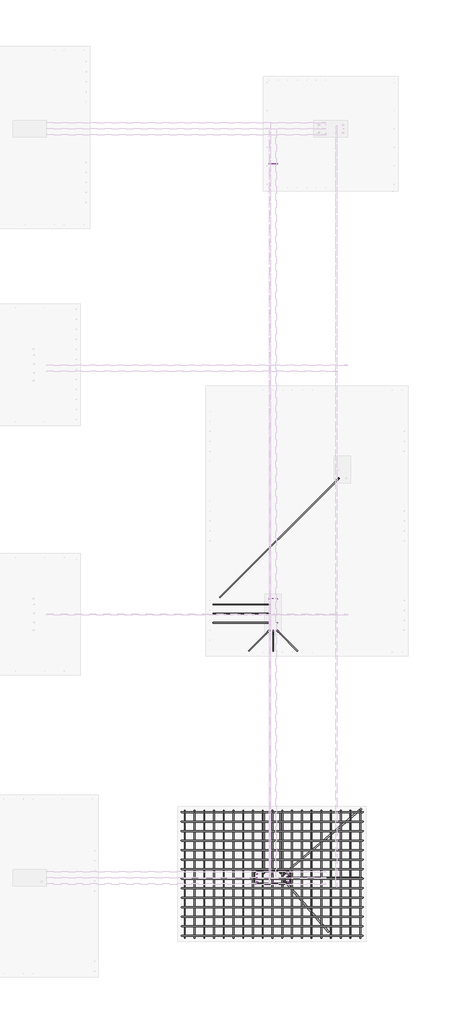
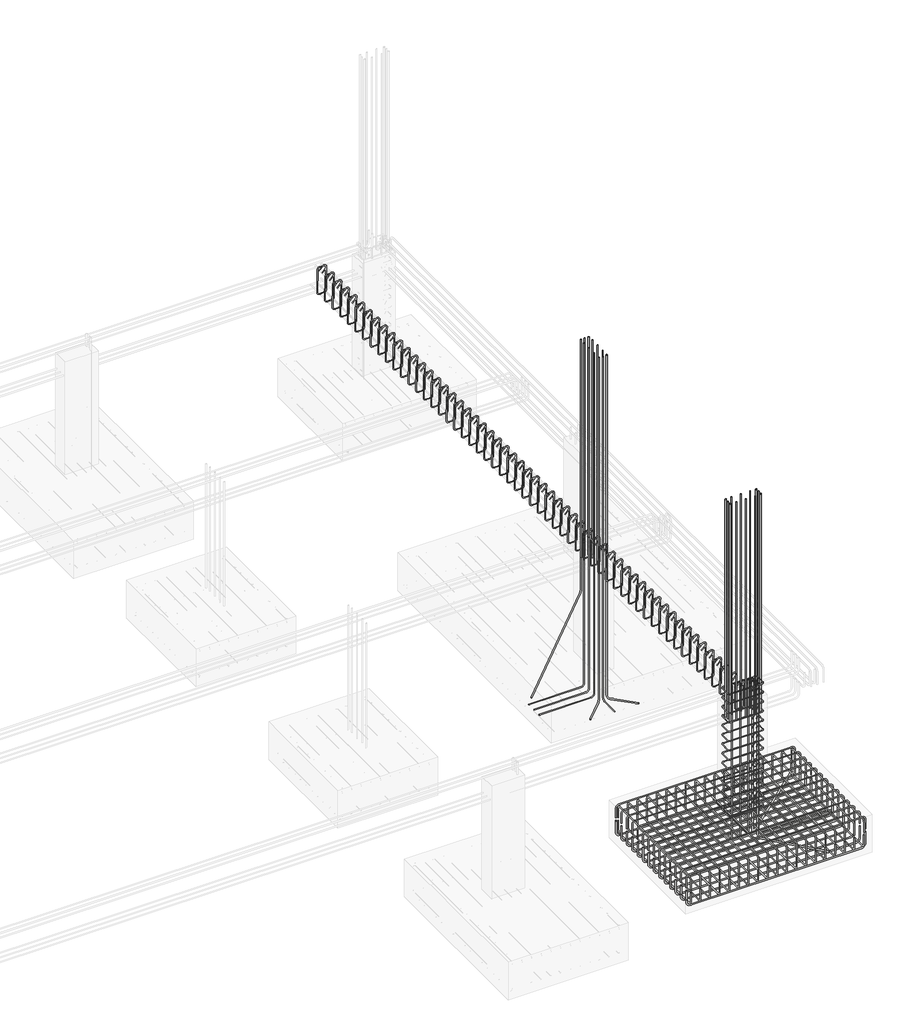
# One storey, part 9 of 18: 31 reinforcing bars.
"""IFC4 building model written with IfcOpenShell, lengths in millimetres."""

from ifc_helpers import new_model, si_unit, point, frame, origin, place, context, project, spatial, polyline, circle_curve, trimmed, segment, composite_curve, source, transform, mapped, element, save
from ifc_brep_helpers import swept_disk

model = new_model("IFC4")

# Units and contexts
model_context = context("Model", 3, world=origin())
ifc_project = project(units=[si_unit("LENGTHUNIT", "METRE", prefix="MILLI")], contexts=[model_context])

# Site, building, storey
site = spatial("IfcSite", under=ifc_project)
building = spatial("IfcBuilding", under=site)
storey = spatial("IfcBuildingStorey", under=building, Elevation=-2000.0)

# Reinforcing bars
placement = place(None, origin())
reinforcing_bar_shape = source(origin(), model_context, "Body", "SolidModel", [
    swept_disk(composite_curve([segment(polyline([(10867.920951, -4585.2975898, -2300.0), (10867.920951, -4585.2975898, -2486.6)]), True, "CONTINUOUS"), segment(trimmed(circle_curve(frame((10812.470951, -4585.2975898, -2486.6), z_axis=(0.0, 1.0, 0.0), x_axis=(55.45000000000073, 0.0, 0.0)), 55.45), [point((10867.920951, -4585.2975898, -2486.6))], [point((10812.470951, -4585.2975898, -2542.05))], True, "CARTESIAN"), True, "CONTINUOUS"), segment(polyline([(10812.470951, -4585.2975898, -2542.05), (8239.270951, -4585.2975898, -2542.05)]), True, "CONTINUOUS"), segment(trimmed(circle_curve(frame((8239.270951, -4585.2975898, -2486.6), z_axis=(0.0, 1.0, 0.0), x_axis=(0.0, 0.0, -55.45000000000027)), 55.45), [point((8239.270951, -4585.2975898, -2542.05))], [point((8183.820951, -4585.2975898, -2486.6))], True, "CARTESIAN"), True, "CONTINUOUS"), segment(polyline([(8183.820951, -4585.2975898, -2486.6), (8183.820951, -4585.2975898, -2300.0)]), True, "CONTINUOUS")], self_intersect=False), 7.95),
])
element("IfcReinforcingBar", 1, at=placement, inside=storey, context=model_context, shape_type="MappedRepresentation", body=[
    mapped(reinforcing_bar_shape, transform((0.0, 0.0, 0.0), x_axis=(1.0, 0.0, 0.0), y_axis=(0.0, 1.0, 0.0), z_axis=(0.0, 0.0, 1.0))),
    mapped(reinforcing_bar_shape, transform((0.0, -140.97506, 0.0), x_axis=(1.0, 0.0, 0.0), y_axis=(0.0, 1.0, 0.0), z_axis=(0.0, 0.0, 1.0))),
    mapped(reinforcing_bar_shape, transform((0.0, -281.9501199, 0.0), x_axis=(1.0, 0.0, 0.0), y_axis=(0.0, 1.0, 0.0), z_axis=(0.0, 0.0, 1.0))),
    mapped(reinforcing_bar_shape, transform((0.0, -422.9251799, 0.0), x_axis=(1.0, 0.0, 0.0), y_axis=(0.0, 1.0, 0.0), z_axis=(0.0, 0.0, 1.0))),
    mapped(reinforcing_bar_shape, transform((0.0, -563.9002399, 0.0), x_axis=(1.0, 0.0, 0.0), y_axis=(0.0, 1.0, 0.0), z_axis=(0.0, 0.0, 1.0))),
    mapped(reinforcing_bar_shape, transform((0.0, -704.8752999, 0.0), x_axis=(1.0, 0.0, 0.0), y_axis=(0.0, 1.0, 0.0), z_axis=(0.0, 0.0, 1.0))),
    mapped(reinforcing_bar_shape, transform((0.0, -845.8503598, 0.0), x_axis=(1.0, 0.0, 0.0), y_axis=(0.0, 1.0, 0.0), z_axis=(0.0, 0.0, 1.0))),
    mapped(reinforcing_bar_shape, transform((0.0, -986.8254198, 0.0), x_axis=(1.0, 0.0, 0.0), y_axis=(0.0, 1.0, 0.0), z_axis=(0.0, 0.0, 1.0))),
    mapped(reinforcing_bar_shape, transform((0.0, -1127.8004798, 0.0), x_axis=(1.0, 0.0, 0.0), y_axis=(0.0, 1.0, 0.0), z_axis=(0.0, 0.0, 1.0))),
    mapped(reinforcing_bar_shape, transform((0.0, -1268.7755397, 0.0), x_axis=(1.0, 0.0, 0.0), y_axis=(0.0, 1.0, 0.0), z_axis=(0.0, 0.0, 1.0))),
    mapped(reinforcing_bar_shape, transform((0.0, -1409.7505997, 0.0), x_axis=(1.0, 0.0, 0.0), y_axis=(0.0, 1.0, 0.0), z_axis=(0.0, 0.0, 1.0))),
    mapped(reinforcing_bar_shape, transform((0.0, -1550.7256597, 0.0), x_axis=(1.0, 0.0, 0.0), y_axis=(0.0, 1.0, 0.0), z_axis=(0.0, 0.0, 1.0))),
    mapped(reinforcing_bar_shape, transform((0.0, -1691.7007197, 0.0), x_axis=(1.0, 0.0, 0.0), y_axis=(0.0, 1.0, 0.0), z_axis=(0.0, 0.0, 1.0))),
    mapped(reinforcing_bar_shape, transform((0.0, -1832.6757796, 0.0), x_axis=(1.0, 0.0, 0.0), y_axis=(0.0, 1.0, 0.0), z_axis=(0.0, 0.0, 1.0))),
])
reinforcing_bar_2_shape = source(origin(), model_context, "Body", "SolidModel", [
    swept_disk(composite_curve([segment(polyline([(8181.870951, -4585.2975898, -2250.0), (8181.870951, -4585.2975898, -2102.0)]), True, "CONTINUOUS"), segment(trimmed(circle_curve(frame((8227.870951, -4585.2975898, -2102.0), z_axis=(0.0, 1.0, 0.0), x_axis=(-46.00000000000091, 0.0, 0.0)), 46.0), [point((8181.870951, -4585.2975898, -2102.0))], [point((8227.870951, -4585.2975898, -2056.0))], True, "CARTESIAN"), True, "CONTINUOUS"), segment(polyline([(8227.870951, -4585.2975898, -2056.0), (10823.870951, -4585.2975898, -2056.0)]), True, "CONTINUOUS"), segment(trimmed(circle_curve(frame((10823.870951, -4585.2975898, -2102.0), z_axis=(0.0, 1.0, 0.0), x_axis=(0.0, 0.0, 46.0)), 46.0), [point((10823.870951, -4585.2975898, -2056.0))], [point((10869.870951, -4585.2975898, -2102.0))], True, "CARTESIAN"), True, "CONTINUOUS"), segment(polyline([(10869.870951, -4585.2975898, -2102.0), (10869.870951, -4585.2975898, -2250.0)]), True, "CONTINUOUS")], self_intersect=False), 6.0),
])
element("IfcReinforcingBar", 2, at=placement, inside=storey, context=model_context, shape_type="MappedRepresentation", body=[
    mapped(reinforcing_bar_2_shape, transform((0.0, 0.0, 0.0), x_axis=(1.0, 0.0, 0.0), y_axis=(0.0, 1.0, 0.0), z_axis=(0.0, 0.0, 1.0))),
    mapped(reinforcing_bar_2_shape, transform((0.0, -140.97506, 0.0), x_axis=(1.0, 0.0, 0.0), y_axis=(0.0, 1.0, 0.0), z_axis=(0.0, 0.0, 1.0))),
    mapped(reinforcing_bar_2_shape, transform((0.0, -281.9501199, 0.0), x_axis=(1.0, 0.0, 0.0), y_axis=(0.0, 1.0, 0.0), z_axis=(0.0, 0.0, 1.0))),
    mapped(reinforcing_bar_2_shape, transform((0.0, -422.9251799, 0.0), x_axis=(1.0, 0.0, 0.0), y_axis=(0.0, 1.0, 0.0), z_axis=(0.0, 0.0, 1.0))),
    mapped(reinforcing_bar_2_shape, transform((0.0, -563.9002399, 0.0), x_axis=(1.0, 0.0, 0.0), y_axis=(0.0, 1.0, 0.0), z_axis=(0.0, 0.0, 1.0))),
    mapped(reinforcing_bar_2_shape, transform((0.0, -704.8752999, 0.0), x_axis=(1.0, 0.0, 0.0), y_axis=(0.0, 1.0, 0.0), z_axis=(0.0, 0.0, 1.0))),
    mapped(reinforcing_bar_2_shape, transform((0.0, -845.8503598, 0.0), x_axis=(1.0, 0.0, 0.0), y_axis=(0.0, 1.0, 0.0), z_axis=(0.0, 0.0, 1.0))),
    mapped(reinforcing_bar_2_shape, transform((0.0, -986.8254198, 0.0), x_axis=(1.0, 0.0, 0.0), y_axis=(0.0, 1.0, 0.0), z_axis=(0.0, 0.0, 1.0))),
    mapped(reinforcing_bar_2_shape, transform((0.0, -1127.8004798, 0.0), x_axis=(1.0, 0.0, 0.0), y_axis=(0.0, 1.0, 0.0), z_axis=(0.0, 0.0, 1.0))),
    mapped(reinforcing_bar_2_shape, transform((0.0, -1268.7755397, 0.0), x_axis=(1.0, 0.0, 0.0), y_axis=(0.0, 1.0, 0.0), z_axis=(0.0, 0.0, 1.0))),
    mapped(reinforcing_bar_2_shape, transform((0.0, -1409.7505997, 0.0), x_axis=(1.0, 0.0, 0.0), y_axis=(0.0, 1.0, 0.0), z_axis=(0.0, 0.0, 1.0))),
    mapped(reinforcing_bar_2_shape, transform((0.0, -1550.7256597, 0.0), x_axis=(1.0, 0.0, 0.0), y_axis=(0.0, 1.0, 0.0), z_axis=(0.0, 0.0, 1.0))),
    mapped(reinforcing_bar_2_shape, transform((0.0, -1691.7007197, 0.0), x_axis=(1.0, 0.0, 0.0), y_axis=(0.0, 1.0, 0.0), z_axis=(0.0, 0.0, 1.0))),
    mapped(reinforcing_bar_2_shape, transform((0.0, -1832.6757796, 0.0), x_axis=(1.0, 0.0, 0.0), y_axis=(0.0, 1.0, 0.0), z_axis=(0.0, 0.0, 1.0))),
])
reinforcing_bar_3_shape = source(origin(), model_context, "Body", "SolidModel", [
    swept_disk(composite_curve([segment(polyline([(8228.0517338, -4562.4021146, -2322.6684255), (8228.0517338, -4562.4021146, -2470.6684255)]), True, "CONTINUOUS"), segment(trimmed(circle_curve(frame((8228.0517338, -4608.4021146, -2470.6684255), z_axis=(-1.0, 0.0, 0.0), x_axis=(0.0, 46.0, 0.0)), 46.0), [point((8228.0517338, -4562.4021146, -2470.6684255))], [point((8228.0517338, -4608.4021146, -2516.6684255))], True, "CARTESIAN"), True, "CONTINUOUS"), segment(polyline([(8228.0517338, -4608.4021146, -2516.6684255), (8228.0517338, -6404.4021146, -2516.6684255)]), True, "CONTINUOUS"), segment(trimmed(circle_curve(frame((8228.0517338, -6404.4021146, -2470.6684255), z_axis=(-1.0, 0.0, 0.0), x_axis=(0.0, 0.0, -46.0)), 46.0), [point((8228.0517338, -6404.4021146, -2516.6684255))], [point((8228.0517338, -6450.4021146, -2470.6684255))], True, "CARTESIAN"), True, "CONTINUOUS"), segment(polyline([(8228.0517338, -6450.4021146, -2470.6684255), (8228.0517338, -6450.4021146, -2322.6684255)]), True, "CONTINUOUS")], self_intersect=False), 6.0),
])
element("IfcReinforcingBar", 3, at=placement, inside=storey, context=model_context, shape_type="MappedRepresentation", body=[
    mapped(reinforcing_bar_3_shape, transform((0.0, 0.0, 0.0), x_axis=(1.0, 0.0, 0.0), y_axis=(0.0, 1.0, 0.0), z_axis=(0.0, 0.0, 1.0))),
    mapped(reinforcing_bar_3_shape, transform((144.6566146, 0.0, 0.0), x_axis=(1.0, 0.0, 0.0), y_axis=(0.0, 1.0, 0.0), z_axis=(0.0, 0.0, 1.0))),
    mapped(reinforcing_bar_3_shape, transform((289.3132291, 0.0, 0.0), x_axis=(1.0, 0.0, 0.0), y_axis=(0.0, 1.0, 0.0), z_axis=(0.0, 0.0, 1.0))),
    mapped(reinforcing_bar_3_shape, transform((433.9698437, 0.0, 0.0), x_axis=(1.0, 0.0, 0.0), y_axis=(0.0, 1.0, 0.0), z_axis=(0.0, 0.0, 1.0))),
    mapped(reinforcing_bar_3_shape, transform((578.6264583, 0.0, 0.0), x_axis=(1.0, 0.0, 0.0), y_axis=(0.0, 1.0, 0.0), z_axis=(0.0, 0.0, 1.0))),
    mapped(reinforcing_bar_3_shape, transform((723.2830729, 0.0, 0.0), x_axis=(1.0, 0.0, 0.0), y_axis=(0.0, 1.0, 0.0), z_axis=(0.0, 0.0, 1.0))),
    mapped(reinforcing_bar_3_shape, transform((867.9396874, 0.0, 0.0), x_axis=(1.0, 0.0, 0.0), y_axis=(0.0, 1.0, 0.0), z_axis=(0.0, 0.0, 1.0))),
    mapped(reinforcing_bar_3_shape, transform((1012.596302, 0.0, 0.0), x_axis=(1.0, 0.0, 0.0), y_axis=(0.0, 1.0, 0.0), z_axis=(0.0, 0.0, 1.0))),
    mapped(reinforcing_bar_3_shape, transform((1157.2529166, 0.0, 0.0), x_axis=(1.0, 0.0, 0.0), y_axis=(0.0, 1.0, 0.0), z_axis=(0.0, 0.0, 1.0))),
    mapped(reinforcing_bar_3_shape, transform((1301.9095312, 0.0, 0.0), x_axis=(1.0, 0.0, 0.0), y_axis=(0.0, 1.0, 0.0), z_axis=(0.0, 0.0, 1.0))),
    mapped(reinforcing_bar_3_shape, transform((1446.5661457, 0.0, 0.0), x_axis=(1.0, 0.0, 0.0), y_axis=(0.0, 1.0, 0.0), z_axis=(0.0, 0.0, 1.0))),
    mapped(reinforcing_bar_3_shape, transform((1591.2227603, 0.0, 0.0), x_axis=(1.0, 0.0, 0.0), y_axis=(0.0, 1.0, 0.0), z_axis=(0.0, 0.0, 1.0))),
    mapped(reinforcing_bar_3_shape, transform((1735.8793749, 0.0, 0.0), x_axis=(1.0, 0.0, 0.0), y_axis=(0.0, 1.0, 0.0), z_axis=(0.0, 0.0, 1.0))),
    mapped(reinforcing_bar_3_shape, transform((1880.5359895, 0.0, 0.0), x_axis=(1.0, 0.0, 0.0), y_axis=(0.0, 1.0, 0.0), z_axis=(0.0, 0.0, 1.0))),
    mapped(reinforcing_bar_3_shape, transform((2025.192604, 0.0, 0.0), x_axis=(1.0, 0.0, 0.0), y_axis=(0.0, 1.0, 0.0), z_axis=(0.0, 0.0, 1.0))),
    mapped(reinforcing_bar_3_shape, transform((2169.8492186, 0.0, 0.0), x_axis=(1.0, 0.0, 0.0), y_axis=(0.0, 1.0, 0.0), z_axis=(0.0, 0.0, 1.0))),
    mapped(reinforcing_bar_3_shape, transform((2314.5058332, 0.0, 0.0), x_axis=(1.0, 0.0, 0.0), y_axis=(0.0, 1.0, 0.0), z_axis=(0.0, 0.0, 1.0))),
    mapped(reinforcing_bar_3_shape, transform((2459.1624478, 0.0, 0.0), x_axis=(1.0, 0.0, 0.0), y_axis=(0.0, 1.0, 0.0), z_axis=(0.0, 0.0, 1.0))),
    mapped(reinforcing_bar_3_shape, transform((2603.8190623, 0.0, 0.0), x_axis=(1.0, 0.0, 0.0), y_axis=(0.0, 1.0, 0.0), z_axis=(0.0, 0.0, 1.0))),
])
reinforcing_bar_4_shape = source(origin(), model_context, "Body", "SolidModel", [
    swept_disk(composite_curve([segment(polyline([(10833.793968, -4562.4021146, -2276.6677805), (10833.793968, -4562.4021146, -2128.6677805)]), True, "CONTINUOUS"), segment(trimmed(circle_curve(frame((10833.793968, -4608.4021146, -2128.6677805), z_axis=(1.0, 0.0, 0.0), x_axis=(0.0, 46.0, 0.0)), 46.0), [point((10833.793968, -4562.4021146, -2128.6677805))], [point((10833.793968, -4608.4021146, -2082.6677805))], True, "CARTESIAN"), True, "CONTINUOUS"), segment(polyline([(10833.793968, -4608.4021146, -2082.6677805), (10833.793968, -6404.4021146, -2082.6677805)]), True, "CONTINUOUS"), segment(trimmed(circle_curve(frame((10833.793968, -6404.4021146, -2128.6677805), z_axis=(1.0, 0.0, 0.0), x_axis=(0.0, 0.0, 46.0)), 46.0), [point((10833.793968, -6404.4021146, -2082.6677805))], [point((10833.793968, -6450.4021146, -2128.6677805))], True, "CARTESIAN"), True, "CONTINUOUS"), segment(polyline([(10833.793968, -6450.4021146, -2128.6677805), (10833.793968, -6450.4021146, -2276.6677805)]), True, "CONTINUOUS")], self_intersect=False), 6.0),
])
element("IfcReinforcingBar", 4, at=placement, inside=storey, context=model_context, shape_type="MappedRepresentation", body=[
    mapped(reinforcing_bar_4_shape, transform((0.0, 0.0, 0.0), x_axis=(1.0, 0.0, 0.0), y_axis=(0.0, 1.0, 0.0), z_axis=(0.0, 0.0, 1.0))),
    mapped(reinforcing_bar_4_shape, transform((-144.7634575, 0.0, 0.0), x_axis=(1.0, 0.0, 0.0), y_axis=(0.0, 1.0, 0.0), z_axis=(0.0, 0.0, 1.0))),
    mapped(reinforcing_bar_4_shape, transform((-289.5269149, 0.0, 0.0), x_axis=(1.0, 0.0, 0.0), y_axis=(0.0, 1.0, 0.0), z_axis=(0.0, 0.0, 1.0))),
    mapped(reinforcing_bar_4_shape, transform((-434.2903724, 0.0, 0.0), x_axis=(1.0, 0.0, 0.0), y_axis=(0.0, 1.0, 0.0), z_axis=(0.0, 0.0, 1.0))),
    mapped(reinforcing_bar_4_shape, transform((-579.0538298, 0.0, 0.0), x_axis=(1.0, 0.0, 0.0), y_axis=(0.0, 1.0, 0.0), z_axis=(0.0, 0.0, 1.0))),
    mapped(reinforcing_bar_4_shape, transform((-723.8172873, 0.0, 0.0), x_axis=(1.0, 0.0, 0.0), y_axis=(0.0, 1.0, 0.0), z_axis=(0.0, 0.0, 1.0))),
    mapped(reinforcing_bar_4_shape, transform((-868.5807447, 0.0, 0.0), x_axis=(1.0, 0.0, 0.0), y_axis=(0.0, 1.0, 0.0), z_axis=(0.0, 0.0, 1.0))),
    mapped(reinforcing_bar_4_shape, transform((-1013.3442022, 0.0, 0.0), x_axis=(1.0, 0.0, 0.0), y_axis=(0.0, 1.0, 0.0), z_axis=(0.0, 0.0, 1.0))),
    mapped(reinforcing_bar_4_shape, transform((-1158.1076596, 0.0, 0.0), x_axis=(1.0, 0.0, 0.0), y_axis=(0.0, 1.0, 0.0), z_axis=(0.0, 0.0, 1.0))),
    mapped(reinforcing_bar_4_shape, transform((-1302.8711171, 0.0, 0.0), x_axis=(1.0, 0.0, 0.0), y_axis=(0.0, 1.0, 0.0), z_axis=(0.0, 0.0, 1.0))),
    mapped(reinforcing_bar_4_shape, transform((-1447.6345745, 0.0, 0.0), x_axis=(1.0, 0.0, 0.0), y_axis=(0.0, 1.0, 0.0), z_axis=(0.0, 0.0, 1.0))),
    mapped(reinforcing_bar_4_shape, transform((-1592.398032, 0.0, 0.0), x_axis=(1.0, 0.0, 0.0), y_axis=(0.0, 1.0, 0.0), z_axis=(0.0, 0.0, 1.0))),
    mapped(reinforcing_bar_4_shape, transform((-1737.1614894, 0.0, 0.0), x_axis=(1.0, 0.0, 0.0), y_axis=(0.0, 1.0, 0.0), z_axis=(0.0, 0.0, 1.0))),
    mapped(reinforcing_bar_4_shape, transform((-1881.9249469, 0.0, 0.0), x_axis=(1.0, 0.0, 0.0), y_axis=(0.0, 1.0, 0.0), z_axis=(0.0, 0.0, 1.0))),
    mapped(reinforcing_bar_4_shape, transform((-2026.6884044, 0.0, 0.0), x_axis=(1.0, 0.0, 0.0), y_axis=(0.0, 1.0, 0.0), z_axis=(0.0, 0.0, 1.0))),
    mapped(reinforcing_bar_4_shape, transform((-2171.4518618, 0.0, 0.0), x_axis=(1.0, 0.0, 0.0), y_axis=(0.0, 1.0, 0.0), z_axis=(0.0, 0.0, 1.0))),
    mapped(reinforcing_bar_4_shape, transform((-2316.2153193, 0.0, 0.0), x_axis=(1.0, 0.0, 0.0), y_axis=(0.0, 1.0, 0.0), z_axis=(0.0, 0.0, 1.0))),
    mapped(reinforcing_bar_4_shape, transform((-2460.9787767, 0.0, 0.0), x_axis=(1.0, 0.0, 0.0), y_axis=(0.0, 1.0, 0.0), z_axis=(0.0, 0.0, 1.0))),
    mapped(reinforcing_bar_4_shape, transform((-2605.7422342, 0.0, 0.0), x_axis=(1.0, 0.0, 0.0), y_axis=(0.0, 1.0, 0.0), z_axis=(0.0, 0.0, 1.0))),
])
reinforcing_bar_5_shape = source(origin(), model_context, "Body", "SolidModel", [
    swept_disk(composite_curve([segment(polyline([(9686.0294026, -5530.2314696, -34.0), (9742.3648543, -5473.8960179, -34.0)]), True, "CONTINUOUS"), segment(trimmed(circle_curve(frame((9762.870951, -5494.4021146, -34.0), z_axis=(0.0, 0.0, -1.0), x_axis=(-20.506096700000853, 20.506096699999944, 0.0)), 29.0), [point((9742.3648543, -5473.8960179, -34.0))], [point((9791.870951, -5494.4021146, -34.0))], True, "CARTESIAN"), True, "CONTINUOUS"), segment(polyline([(9791.870951, -5494.4021146, -34.0), (9791.870951, -5618.4021146, -34.0)]), True, "CONTINUOUS"), segment(trimmed(circle_curve(frame((9762.870951, -5618.4021146, -34.0), z_axis=(0.0, 0.0, -1.0), x_axis=(29.0, 0.0, 0.0)), 29.0), [point((9791.870951, -5618.4021146, -34.0))], [point((9762.870951, -5647.4021146, -34.0))], True, "CARTESIAN"), True, "CONTINUOUS"), segment(polyline([(9762.870951, -5647.4021146, -34.0), (9288.870951, -5647.4021146, -34.0)]), True, "CONTINUOUS"), segment(trimmed(circle_curve(frame((9288.870951, -5618.43009, -32.7265044), z_axis=(0.0, 0.043913640913297095, -0.9990353307775146), x_axis=(0.0, -28.972024599999713, -1.2734955999999968)), 29.0), [point((9288.870951, -5647.4021146, -34.0))], [point((9259.870951, -5618.43009, -32.7265044))], True, "CARTESIAN"), True, "CONTINUOUS"), segment(polyline([(9259.870951, -5618.43009, -32.7265044), (9259.870951, -5494.3741392, -27.2734956)]), True, "CONTINUOUS"), segment(trimmed(circle_curve(frame((9288.870951, -5494.3741392, -27.2734956), z_axis=(0.0, 0.043913640913297095, -0.9990353307775146), x_axis=(-29.0, 0.0, 0.0)), 29.0), [point((9259.870951, -5494.3741392, -27.2734956))], [point((9288.870951, -5465.4021146, -26.0))], True, "CARTESIAN"), True, "CONTINUOUS"), segment(polyline([(9288.870951, -5465.4021146, -26.0), (9762.870951, -5465.4021146, -26.0)]), True, "CONTINUOUS"), segment(trimmed(circle_curve(frame((9762.870951, -5494.4021146, -26.0), z_axis=(0.0, 0.0, -1.0), x_axis=(0.0, 29.0, 0.0)), 29.0), [point((9762.870951, -5465.4021146, -26.0))], [point((9783.3770476, -5514.9082112, -26.0))], True, "CARTESIAN"), True, "CONTINUOUS"), segment(polyline([(9783.3770476, -5514.9082112, -26.0), (9727.041596, -5571.2436629, -26.0)]), True, "CONTINUOUS")], self_intersect=False), 4.0),
])
element("IfcReinforcingBar", 5, at=placement, inside=storey, context=model_context, shape_type="MappedRepresentation", body=[
    mapped(reinforcing_bar_5_shape, transform((0.0, 0.0, 0.0), x_axis=(1.0, 0.0, 0.0), y_axis=(0.0, 1.0, 0.0), z_axis=(0.0, 0.0, 1.0))),
    mapped(reinforcing_bar_5_shape, transform((0.0, 0.0, -148.6153846), x_axis=(1.0, 0.0, 0.0), y_axis=(0.0, 1.0, 0.0), z_axis=(0.0, 0.0, 1.0))),
    mapped(reinforcing_bar_5_shape, transform((0.0, 0.0, -297.2307692), x_axis=(1.0, 0.0, 0.0), y_axis=(0.0, 1.0, 0.0), z_axis=(0.0, 0.0, 1.0))),
    mapped(reinforcing_bar_5_shape, transform((0.0, 0.0, -445.8461538), x_axis=(1.0, 0.0, 0.0), y_axis=(0.0, 1.0, 0.0), z_axis=(0.0, 0.0, 1.0))),
    mapped(reinforcing_bar_5_shape, transform((0.0, 0.0, -594.4615385), x_axis=(1.0, 0.0, 0.0), y_axis=(0.0, 1.0, 0.0), z_axis=(0.0, 0.0, 1.0))),
    mapped(reinforcing_bar_5_shape, transform((0.0, 0.0, -743.0769231), x_axis=(1.0, 0.0, 0.0), y_axis=(0.0, 1.0, 0.0), z_axis=(0.0, 0.0, 1.0))),
    mapped(reinforcing_bar_5_shape, transform((0.0, 0.0, -891.6923077), x_axis=(1.0, 0.0, 0.0), y_axis=(0.0, 1.0, 0.0), z_axis=(0.0, 0.0, 1.0))),
    mapped(reinforcing_bar_5_shape, transform((0.0, 0.0, -1040.3076923), x_axis=(1.0, 0.0, 0.0), y_axis=(0.0, 1.0, 0.0), z_axis=(0.0, 0.0, 1.0))),
    mapped(reinforcing_bar_5_shape, transform((0.0, 0.0, -1188.9230769), x_axis=(1.0, 0.0, 0.0), y_axis=(0.0, 1.0, 0.0), z_axis=(0.0, 0.0, 1.0))),
    mapped(reinforcing_bar_5_shape, transform((0.0, 0.0, -1337.5384615), x_axis=(1.0, 0.0, 0.0), y_axis=(0.0, 1.0, 0.0), z_axis=(0.0, 0.0, 1.0))),
    mapped(reinforcing_bar_5_shape, transform((0.0, 0.0, -1486.1538462), x_axis=(1.0, 0.0, 0.0), y_axis=(0.0, 1.0, 0.0), z_axis=(0.0, 0.0, 1.0))),
    mapped(reinforcing_bar_5_shape, transform((0.0, 0.0, -1634.7692308), x_axis=(1.0, 0.0, 0.0), y_axis=(0.0, 1.0, 0.0), z_axis=(0.0, 0.0, 1.0))),
    mapped(reinforcing_bar_5_shape, transform((0.0, 0.0, -1783.3846154), x_axis=(1.0, 0.0, 0.0), y_axis=(0.0, 1.0, 0.0), z_axis=(0.0, 0.0, 1.0))),
    mapped(reinforcing_bar_5_shape, transform((0.0, 0.0, -1932.0), x_axis=(1.0, 0.0, 0.0), y_axis=(0.0, 1.0, 0.0), z_axis=(0.0, 0.0, 1.0))),
])
element("IfcReinforcingBar", 6, at=placement, inside=storey, context=model_context, shape_type="SolidModel", body=[
    swept_disk(composite_curve([segment(polyline([(10849.1502881, -4537.960597, -2480.0), (9755.7367866, -5455.4434628, -2480.0)]), True, "CONTINUOUS"), segment(trimmed(circle_curve(frame((9755.7367866, -5455.4434628, -2412.5), z_axis=(-0.6427876096865429, 0.766044443118975, 0.0), x_axis=(0.0, 0.0, -67.5)), 67.5), [point((9755.7367866, -5455.4434628, -2480.0))], [point((9704.0287867, -5498.8316264, -2412.5))], True, "CARTESIAN"), True, "CONTINUOUS"), segment(polyline([(9704.0287867, -5498.8316264, -2412.5), (9704.0287867, -5498.8316264, -20.0)]), True, "CONTINUOUS")], self_intersect=False), 10.0),
])
element("IfcReinforcingBar", 7, at=placement, inside=storey, context=model_context, shape_type="SolidModel", body=[
    swept_disk(composite_curve([segment(polyline([(10361.8457458, -6359.2007661, -2480.0), (9758.3127712, -5664.9154994, -2480.0)]), True, "CONTINUOUS"), segment(trimmed(circle_curve(frame((9758.3127712, -5664.9154994, -2412.5), z_axis=(0.7547095802227678, 0.6560590289905122, 0.0), x_axis=(0.0, 0.0, -67.5)), 67.5), [point((9758.3127712, -5664.9154994, -2480.0))], [point((9714.0287867, -5613.9726027, -2412.5))], True, "CARTESIAN"), True, "CONTINUOUS"), segment(polyline([(9714.0287867, -5613.9726027, -2412.5), (9714.0287867, -5613.9726027, -20.0)]), True, "CONTINUOUS")], self_intersect=False), 10.0),
])
element("IfcReinforcingBar", 8, at=placement, inside=storey, context=model_context, shape_type="SolidModel", body=[
    swept_disk(composite_curve([segment(polyline([(10853.1846074, -5554.0856321, -2480.0), (9810.3889128, -5554.0856321, -2480.0)]), True, "CONTINUOUS"), segment(trimmed(circle_curve(frame((9810.3889128, -5554.0856321, -2434.0), z_axis=(0.0, 1.0, 0.0), x_axis=(0.0, 0.0, -46.0)), 46.0), [point((9810.3889128, -5554.0856321, -2480.0))], [point((9764.3889128, -5554.0856321, -2434.0))], True, "CARTESIAN"), True, "CONTINUOUS"), segment(polyline([(9764.3889128, -5554.0856321, -2434.0), (9764.3889128, -5554.0856321, -30.0)]), True, "CONTINUOUS")], self_intersect=False), 6.0),
])
reinforcing_bar_6_shape = source(origin(), model_context, "Body", "SolidModel", [
    swept_disk(composite_curve([segment(polyline([(9402.8188559, -4586.3567, -2480.0), (9402.8188559, -5444.3642821, -2480.0)]), True, "CONTINUOUS"), segment(trimmed(circle_curve(frame((9402.8188559, -5444.3642821, -2434.0), z_axis=(-1.0, 0.0, 0.0), x_axis=(0.0, 0.0, -46.0)), 46.0), [point((9402.8188559, -5444.3642821, -2480.0))], [point((9402.8188559, -5490.3642821, -2434.0))], True, "CARTESIAN"), True, "CONTINUOUS"), segment(polyline([(9402.8188559, -5490.3642821, -2434.0), (9402.8188559, -5490.3642821, -30.0)]), True, "CONTINUOUS")], self_intersect=False), 6.0),
])
element("IfcReinforcingBar", 9, at=placement, inside=storey, context=model_context, shape_type="MappedRepresentation", body=[
    mapped(reinforcing_bar_6_shape, transform((0.0, 0.0, 0.0), x_axis=(1.0, 0.0, 0.0), y_axis=(0.0, 1.0, 0.0), z_axis=(0.0, 0.0, 1.0))),
    mapped(reinforcing_bar_6_shape, transform((122.4797009, 0.0, 0.0), x_axis=(1.0, 0.0, 0.0), y_axis=(0.0, 1.0, 0.0), z_axis=(0.0, 0.0, 1.0))),
    mapped(reinforcing_bar_6_shape, transform((244.9594019, 0.0, 0.0), x_axis=(1.0, 0.0, 0.0), y_axis=(0.0, 1.0, 0.0), z_axis=(0.0, 0.0, 1.0))),
])
reinforcing_bar_7_shape = source(origin(), model_context, "Body", "SolidModel", [
    swept_disk(composite_curve([segment(polyline([(9475.7493386, -1776.5422299, -30.0), (9475.7493386, -1776.5422299, -2436.6982733)]), True, "CONTINUOUS"), segment(trimmed(circle_curve(frame((9429.7493386, -1776.5422299, -2436.6982733), z_axis=(0.0, 1.0, 0.0), x_axis=(46.0, 0.0, 0.0)), 46.0), [point((9475.7493386, -1776.5422299, -2436.6982733))], [point((9429.7493386, -1776.5422299, -2482.6982733))], True, "CARTESIAN"), True, "CONTINUOUS"), segment(polyline([(9429.7493386, -1776.5422299, -2482.6982733), (8648.7341226, -1776.5422299, -2482.6982733)]), True, "CONTINUOUS")], self_intersect=False), 6.0),
])
element("IfcReinforcingBar", 10, at=placement, inside=storey, context=model_context, shape_type="MappedRepresentation", body=[
    mapped(reinforcing_bar_7_shape, transform((0.0, 0.0, 0.0), x_axis=(1.0, 0.0, 0.0), y_axis=(0.0, 1.0, 0.0), z_axis=(0.0, 0.0, 1.0))),
    mapped(reinforcing_bar_7_shape, transform((0.0, 134.2724138, 0.0), x_axis=(1.0, 0.0, 0.0), y_axis=(0.0, 1.0, 0.0), z_axis=(0.0, 0.0, 1.0))),
    mapped(reinforcing_bar_7_shape, transform((0.0, 268.5448277, 0.0), x_axis=(1.0, 0.0, 0.0), y_axis=(0.0, 1.0, 0.0), z_axis=(0.0, 0.0, 1.0))),
])
element("IfcReinforcingBar", 11, at=placement, inside=storey, context=model_context, shape_type="SolidModel", body=[
    swept_disk(composite_curve([segment(polyline([(9539.2080766, -1896.3217695, -30.0), (9539.2080766, -1896.3217695, -2440.6)]), True, "CONTINUOUS"), segment(trimmed(circle_curve(frame((9539.2080766, -1942.3217695, -2440.6), z_axis=(-1.0, 0.0, 0.0), x_axis=(0.0, 46.0, 0.0)), 46.0), [point((9539.2080766, -1896.3217695, -2440.6))], [point((9539.2080766, -1942.3217695, -2486.6))], True, "CARTESIAN"), True, "CONTINUOUS"), segment(polyline([(9539.2080766, -1942.3217695, -2486.6), (9539.2080766, -2198.8907934, -2486.6)]), True, "CONTINUOUS")], self_intersect=False), 6.0),
])
element("IfcReinforcingBar", 12, at=placement, inside=storey, context=model_context, shape_type="SolidModel", body=[
    swept_disk(composite_curve([segment(polyline([(9481.9100581, -1891.7202311, -30.0), (9481.9100581, -1891.7202311, -2431.15)]), True, "CONTINUOUS"), segment(trimmed(circle_curve(frame((9442.7009871, -1930.9293021, -2431.15), z_axis=(-0.7071067811865454, 0.7071067811865497, 0.0), x_axis=(39.20907100000113, 39.209070999999994, 0.0)), 55.45), [point((9481.9100581, -1891.7202311, -2431.15))], [point((9442.7009871, -1930.9293021, -2486.6))], True, "CARTESIAN"), True, "CONTINUOUS"), segment(polyline([(9442.7009871, -1930.9293021, -2486.6), (9177.9135965, -2195.7166928, -2486.6)]), True, "CONTINUOUS")], self_intersect=False), 7.95),
])
element("IfcReinforcingBar", 13, at=placement, inside=storey, context=model_context, shape_type="SolidModel", body=[
    swept_disk(composite_curve([segment(polyline([(9597.4019305, -1891.7202311, -30.0), (9597.4019305, -1891.7202311, -2431.15)]), True, "CONTINUOUS"), segment(trimmed(circle_curve(frame((9636.6110015, -1930.9293021, -2431.15), z_axis=(-0.7071067811865546, -0.7071067811865406, 0.0), x_axis=(-39.20907099999931, 39.209070999999994, 0.0)), 55.45), [point((9597.4019305, -1891.7202311, -2431.15))], [point((9636.6110015, -1930.9293021, -2486.6))], True, "CARTESIAN"), True, "CONTINUOUS"), segment(polyline([(9636.6110015, -1930.9293021, -2486.6), (9901.3983921, -2195.7166928, -2486.6)]), True, "CONTINUOUS")], self_intersect=False), 7.95),
])
element("IfcReinforcingBar", 14, at=placement, inside=storey, context=model_context, shape_type="SolidModel", body=[
    swept_disk(composite_curve([segment(polyline([(10512.4455347, 360.8875728, -30.0), (10512.4455347, 360.8875728, -2415.2184255)]), True, "CONTINUOUS"), segment(trimmed(circle_curve(frame((10473.2364637, 321.6785018, -2415.2184255), z_axis=(-0.7071067811865474, 0.7071067811865478, 0.0), x_axis=(39.20907100000113, 39.209070999999994, 0.0)), 55.45), [point((10512.4455347, 360.8875728, -2415.2184255))], [point((10473.2364637, 321.6785018, -2470.6684255))], True, "CARTESIAN"), True, "CONTINUOUS"), segment(polyline([(10473.2364637, 321.6785018, -2470.6684255), (8748.0164151, -1403.5415468, -2470.6684255)]), True, "CONTINUOUS")], self_intersect=False), 7.95),
])
reinforcing_bar_8_shape = source(origin(), model_context, "Body", "SolidModel", [
    swept_disk(composite_curve([segment(polyline([(9499.814446, -5445.6797656, -98.829355), (9556.1498976, -5445.6797656, -42.4939033)]), True, "CONTINUOUS"), segment(trimmed(circle_curve(frame((9576.6559943, -5445.6797656, -63.0), z_axis=(0.0, 1.0, 0.0), x_axis=(-20.506096699999034, 0.0, 20.5060967)), 29.0), [point((9556.1498976, -5445.6797656, -42.4939033))], [point((9605.6559943, -5445.6797656, -63.0))], True, "CARTESIAN"), True, "CONTINUOUS"), segment(polyline([(9605.6559943, -5445.6797656, -63.0), (9605.6559943, -5445.6797656, -437.0)]), True, "CONTINUOUS"), segment(trimmed(circle_curve(frame((9576.6559943, -5445.6797656, -437.0), z_axis=(0.0, 1.0, 0.0), x_axis=(29.0, 0.0, 0.0)), 29.0), [point((9605.6559943, -5445.6797656, -437.0))], [point((9576.6559943, -5445.6797656, -466.0))], True, "CARTESIAN"), True, "CONTINUOUS"), segment(polyline([(9576.6559943, -5445.6797656, -466.0), (9502.6559943, -5445.6797656, -466.0)]), True, "CONTINUOUS"), segment(trimmed(circle_curve(frame((9502.6559943, -5446.2167105, -437.0049713), z_axis=(0.0, 0.9998285763251312, 0.018515344006020954), x_axis=(0.0, 0.5369448999999804, -28.995028699999978)), 29.0), [point((9502.6559943, -5445.6797656, -466.0))], [point((9473.6559943, -5446.2167105, -437.0049713))], True, "CARTESIAN"), True, "CONTINUOUS"), segment(polyline([(9473.6559943, -5446.2167105, -437.0049713), (9473.6559943, -5453.1428206, -62.9950287)]), True, "CONTINUOUS"), segment(trimmed(circle_curve(frame((9502.6559943, -5453.1428206, -62.9950287), z_axis=(0.0, 0.9998285763251312, 0.018515344006020954), x_axis=(-29.0, 0.0, 0.0)), 29.0), [point((9473.6559943, -5453.1428206, -62.9950287))], [point((9502.6559943, -5453.6797656, -34.0))], True, "CARTESIAN"), True, "CONTINUOUS"), segment(polyline([(9502.6559943, -5453.6797656, -34.0), (9576.6559943, -5453.6797656, -34.0)]), True, "CONTINUOUS"), segment(trimmed(circle_curve(frame((9576.6559943, -5453.6797656, -63.0), z_axis=(0.0, 1.0, 0.0), x_axis=(0.0, 0.0, 29.0)), 29.0), [point((9576.6559943, -5453.6797656, -34.0))], [point((9597.162091, -5453.6797656, -83.5060967))], True, "CARTESIAN"), True, "CONTINUOUS"), segment(polyline([(9597.162091, -5453.6797656, -83.5060967), (9540.8266393, -5453.6797656, -139.8415483)]), True, "CONTINUOUS")], self_intersect=False), 4.0),
])
element("IfcReinforcingBar", 15, at=placement, inside=storey, context=model_context, shape_type="MappedRepresentation", body=[
    mapped(reinforcing_bar_8_shape, transform((0.0, 0.0, 0.0), x_axis=(1.0, 0.0, 0.0), y_axis=(0.0, 1.0, 0.0), z_axis=(0.0, 0.0, 1.0))),
    mapped(reinforcing_bar_8_shape, transform((0.0, 197.6777755, 0.0), x_axis=(1.0, 0.0, 0.0), y_axis=(0.0, 1.0, 0.0), z_axis=(0.0, 0.0, 1.0))),
    mapped(reinforcing_bar_8_shape, transform((0.0, 395.3555509, 0.0), x_axis=(1.0, 0.0, 0.0), y_axis=(0.0, 1.0, 0.0), z_axis=(0.0, 0.0, 1.0))),
    mapped(reinforcing_bar_8_shape, transform((0.0, 593.0333264, 0.0), x_axis=(1.0, 0.0, 0.0), y_axis=(0.0, 1.0, 0.0), z_axis=(0.0, 0.0, 1.0))),
    mapped(reinforcing_bar_8_shape, transform((0.0, 790.7111019, 0.0), x_axis=(1.0, 0.0, 0.0), y_axis=(0.0, 1.0, 0.0), z_axis=(0.0, 0.0, 1.0))),
    mapped(reinforcing_bar_8_shape, transform((0.0, 988.3888774, 0.0), x_axis=(1.0, 0.0, 0.0), y_axis=(0.0, 1.0, 0.0), z_axis=(0.0, 0.0, 1.0))),
    mapped(reinforcing_bar_8_shape, transform((0.0, 1186.0666528, 0.0), x_axis=(1.0, 0.0, 0.0), y_axis=(0.0, 1.0, 0.0), z_axis=(0.0, 0.0, 1.0))),
    mapped(reinforcing_bar_8_shape, transform((0.0, 1383.7444283, 0.0), x_axis=(1.0, 0.0, 0.0), y_axis=(0.0, 1.0, 0.0), z_axis=(0.0, 0.0, 1.0))),
    mapped(reinforcing_bar_8_shape, transform((0.0, 1581.4222038, 0.0), x_axis=(1.0, 0.0, 0.0), y_axis=(0.0, 1.0, 0.0), z_axis=(0.0, 0.0, 1.0))),
    mapped(reinforcing_bar_8_shape, transform((0.0, 1779.0999793, 0.0), x_axis=(1.0, 0.0, 0.0), y_axis=(0.0, 1.0, 0.0), z_axis=(0.0, 0.0, 1.0))),
    mapped(reinforcing_bar_8_shape, transform((0.0, 1976.7777547, 0.0), x_axis=(1.0, 0.0, 0.0), y_axis=(0.0, 1.0, 0.0), z_axis=(0.0, 0.0, 1.0))),
    mapped(reinforcing_bar_8_shape, transform((0.0, 2174.4555302, 0.0), x_axis=(1.0, 0.0, 0.0), y_axis=(0.0, 1.0, 0.0), z_axis=(0.0, 0.0, 1.0))),
    mapped(reinforcing_bar_8_shape, transform((0.0, 2372.1333057, 0.0), x_axis=(1.0, 0.0, 0.0), y_axis=(0.0, 1.0, 0.0), z_axis=(0.0, 0.0, 1.0))),
    mapped(reinforcing_bar_8_shape, transform((0.0, 2569.8110811, 0.0), x_axis=(1.0, 0.0, 0.0), y_axis=(0.0, 1.0, 0.0), z_axis=(0.0, 0.0, 1.0))),
    mapped(reinforcing_bar_8_shape, transform((0.0, 2767.4888566, 0.0), x_axis=(1.0, 0.0, 0.0), y_axis=(0.0, 1.0, 0.0), z_axis=(0.0, 0.0, 1.0))),
    mapped(reinforcing_bar_8_shape, transform((0.0, 2965.1666321, 0.0), x_axis=(1.0, 0.0, 0.0), y_axis=(0.0, 1.0, 0.0), z_axis=(0.0, 0.0, 1.0))),
    mapped(reinforcing_bar_8_shape, transform((0.0, 3162.8444076, 0.0), x_axis=(1.0, 0.0, 0.0), y_axis=(0.0, 1.0, 0.0), z_axis=(0.0, 0.0, 1.0))),
    mapped(reinforcing_bar_8_shape, transform((0.0, 3360.522183, 0.0), x_axis=(1.0, 0.0, 0.0), y_axis=(0.0, 1.0, 0.0), z_axis=(0.0, 0.0, 1.0))),
    mapped(reinforcing_bar_8_shape, transform((0.0, 3558.1999585, 0.0), x_axis=(1.0, 0.0, 0.0), y_axis=(0.0, 1.0, 0.0), z_axis=(0.0, 0.0, 1.0))),
    mapped(reinforcing_bar_8_shape, transform((0.0, 3755.877734, 0.0), x_axis=(1.0, 0.0, 0.0), y_axis=(0.0, 1.0, 0.0), z_axis=(0.0, 0.0, 1.0))),
    mapped(reinforcing_bar_8_shape, transform((0.0, 3953.5555094, 0.0), x_axis=(1.0, 0.0, 0.0), y_axis=(0.0, 1.0, 0.0), z_axis=(0.0, 0.0, 1.0))),
    mapped(reinforcing_bar_8_shape, transform((0.0, 4151.2332849, 0.0), x_axis=(1.0, 0.0, 0.0), y_axis=(0.0, 1.0, 0.0), z_axis=(0.0, 0.0, 1.0))),
    mapped(reinforcing_bar_8_shape, transform((0.0, 4348.9110604, 0.0), x_axis=(1.0, 0.0, 0.0), y_axis=(0.0, 1.0, 0.0), z_axis=(0.0, 0.0, 1.0))),
    mapped(reinforcing_bar_8_shape, transform((0.0, 4546.5888359, 0.0), x_axis=(1.0, 0.0, 0.0), y_axis=(0.0, 1.0, 0.0), z_axis=(0.0, 0.0, 1.0))),
    mapped(reinforcing_bar_8_shape, transform((0.0, 4744.2666113, 0.0), x_axis=(1.0, 0.0, 0.0), y_axis=(0.0, 1.0, 0.0), z_axis=(0.0, 0.0, 1.0))),
    mapped(reinforcing_bar_8_shape, transform((0.0, 4941.9443868, 0.0), x_axis=(1.0, 0.0, 0.0), y_axis=(0.0, 1.0, 0.0), z_axis=(0.0, 0.0, 1.0))),
    mapped(reinforcing_bar_8_shape, transform((0.0, 5139.6221623, 0.0), x_axis=(1.0, 0.0, 0.0), y_axis=(0.0, 1.0, 0.0), z_axis=(0.0, 0.0, 1.0))),
    mapped(reinforcing_bar_8_shape, transform((0.0, 5337.2999378, 0.0), x_axis=(1.0, 0.0, 0.0), y_axis=(0.0, 1.0, 0.0), z_axis=(0.0, 0.0, 1.0))),
    mapped(reinforcing_bar_8_shape, transform((0.0, 5534.9777132, 0.0), x_axis=(1.0, 0.0, 0.0), y_axis=(0.0, 1.0, 0.0), z_axis=(0.0, 0.0, 1.0))),
    mapped(reinforcing_bar_8_shape, transform((0.0, 5732.6554887, 0.0), x_axis=(1.0, 0.0, 0.0), y_axis=(0.0, 1.0, 0.0), z_axis=(0.0, 0.0, 1.0))),
    mapped(reinforcing_bar_8_shape, transform((0.0, 5930.3332642, 0.0), x_axis=(1.0, 0.0, 0.0), y_axis=(0.0, 1.0, 0.0), z_axis=(0.0, 0.0, 1.0))),
    mapped(reinforcing_bar_8_shape, transform((0.0, 6128.0110396, 0.0), x_axis=(1.0, 0.0, 0.0), y_axis=(0.0, 1.0, 0.0), z_axis=(0.0, 0.0, 1.0))),
    mapped(reinforcing_bar_8_shape, transform((0.0, 6325.6888151, 0.0), x_axis=(1.0, 0.0, 0.0), y_axis=(0.0, 1.0, 0.0), z_axis=(0.0, 0.0, 1.0))),
    mapped(reinforcing_bar_8_shape, transform((0.0, 6523.3665906, 0.0), x_axis=(1.0, 0.0, 0.0), y_axis=(0.0, 1.0, 0.0), z_axis=(0.0, 0.0, 1.0))),
    mapped(reinforcing_bar_8_shape, transform((0.0, 6721.0443661, 0.0), x_axis=(1.0, 0.0, 0.0), y_axis=(0.0, 1.0, 0.0), z_axis=(0.0, 0.0, 1.0))),
    mapped(reinforcing_bar_8_shape, transform((0.0, 6918.7221415, 0.0), x_axis=(1.0, 0.0, 0.0), y_axis=(0.0, 1.0, 0.0), z_axis=(0.0, 0.0, 1.0))),
    mapped(reinforcing_bar_8_shape, transform((0.0, 7116.399917, 0.0), x_axis=(1.0, 0.0, 0.0), y_axis=(0.0, 1.0, 0.0), z_axis=(0.0, 0.0, 1.0))),
    mapped(reinforcing_bar_8_shape, transform((0.0, 7314.0776925, 0.0), x_axis=(1.0, 0.0, 0.0), y_axis=(0.0, 1.0, 0.0), z_axis=(0.0, 0.0, 1.0))),
    mapped(reinforcing_bar_8_shape, transform((0.0, 7511.7554679, 0.0), x_axis=(1.0, 0.0, 0.0), y_axis=(0.0, 1.0, 0.0), z_axis=(0.0, 0.0, 1.0))),
    mapped(reinforcing_bar_8_shape, transform((0.0, 7709.4332434, 0.0), x_axis=(1.0, 0.0, 0.0), y_axis=(0.0, 1.0, 0.0), z_axis=(0.0, 0.0, 1.0))),
    mapped(reinforcing_bar_8_shape, transform((0.0, 7907.1110189, 0.0), x_axis=(1.0, 0.0, 0.0), y_axis=(0.0, 1.0, 0.0), z_axis=(0.0, 0.0, 1.0))),
    mapped(reinforcing_bar_8_shape, transform((0.0, 8104.7887944, 0.0), x_axis=(1.0, 0.0, 0.0), y_axis=(0.0, 1.0, 0.0), z_axis=(0.0, 0.0, 1.0))),
    mapped(reinforcing_bar_8_shape, transform((0.0, 8302.4665698, 0.0), x_axis=(1.0, 0.0, 0.0), y_axis=(0.0, 1.0, 0.0), z_axis=(0.0, 0.0, 1.0))),
    mapped(reinforcing_bar_8_shape, transform((0.0, 8500.1443453, 0.0), x_axis=(1.0, 0.0, 0.0), y_axis=(0.0, 1.0, 0.0), z_axis=(0.0, 0.0, 1.0))),
    mapped(reinforcing_bar_8_shape, transform((0.0, 8697.8221208, 0.0), x_axis=(1.0, 0.0, 0.0), y_axis=(0.0, 1.0, 0.0), z_axis=(0.0, 0.0, 1.0))),
    mapped(reinforcing_bar_8_shape, transform((0.0, 8895.4998963, 0.0), x_axis=(1.0, 0.0, 0.0), y_axis=(0.0, 1.0, 0.0), z_axis=(0.0, 0.0, 1.0))),
    mapped(reinforcing_bar_8_shape, transform((0.0, 9093.1776717, 0.0), x_axis=(1.0, 0.0, 0.0), y_axis=(0.0, 1.0, 0.0), z_axis=(0.0, 0.0, 1.0))),
    mapped(reinforcing_bar_8_shape, transform((0.0, 9290.8554472, 0.0), x_axis=(1.0, 0.0, 0.0), y_axis=(0.0, 1.0, 0.0), z_axis=(0.0, 0.0, 1.0))),
    mapped(reinforcing_bar_8_shape, transform((0.0, 9488.5332227, 0.0), x_axis=(1.0, 0.0, 0.0), y_axis=(0.0, 1.0, 0.0), z_axis=(0.0, 0.0, 1.0))),
    mapped(reinforcing_bar_8_shape, transform((0.0, 9686.2109981, 0.0), x_axis=(1.0, 0.0, 0.0), y_axis=(0.0, 1.0, 0.0), z_axis=(0.0, 0.0, 1.0))),
    mapped(reinforcing_bar_8_shape, transform((0.0, 9883.8887736, 0.0), x_axis=(1.0, 0.0, 0.0), y_axis=(0.0, 1.0, 0.0), z_axis=(0.0, 0.0, 1.0))),
    mapped(reinforcing_bar_8_shape, transform((0.0, 10081.5665491, 0.0), x_axis=(1.0, 0.0, 0.0), y_axis=(0.0, 1.0, 0.0), z_axis=(0.0, 0.0, 1.0))),
    mapped(reinforcing_bar_8_shape, transform((0.0, 10279.2443246, 0.0), x_axis=(1.0, 0.0, 0.0), y_axis=(0.0, 1.0, 0.0), z_axis=(0.0, 0.0, 1.0))),
    mapped(reinforcing_bar_8_shape, transform((0.0, 10476.9221, 0.0), x_axis=(1.0, 0.0, 0.0), y_axis=(0.0, 1.0, 0.0), z_axis=(0.0, 0.0, 1.0))),
    mapped(reinforcing_bar_8_shape, transform((0.0, 10674.5998755, 0.0), x_axis=(1.0, 0.0, 0.0), y_axis=(0.0, 1.0, 0.0), z_axis=(0.0, 0.0, 1.0))),
    mapped(reinforcing_bar_8_shape, transform((0.0, 10872.277651, 0.0), x_axis=(1.0, 0.0, 0.0), y_axis=(0.0, 1.0, 0.0), z_axis=(0.0, 0.0, 1.0))),
])
element("IfcReinforcingBar", 16, at=placement, inside=storey, context=model_context, shape_type="SolidModel", body=[
    swept_disk(composite_curve([segment(polyline([(9481.6640946, -1423.0839981, 2970.0), (9481.6640946, -1423.0839981, -486.6)]), True, "CONTINUOUS")], self_intersect=False), 7.95),
])
element("IfcReinforcingBar", 17, at=placement, inside=storey, context=model_context, shape_type="SolidModel", body=[
    swept_disk(composite_curve([segment(polyline([(9538.962113, -1418.4824597, 2970.0), (9538.962113, -1418.4824597, -486.6)]), True, "CONTINUOUS")], self_intersect=False), 6.0),
])
reinforcing_bar_9_shape = source(origin(), model_context, "Body", "SolidModel", [
    swept_disk(composite_curve([segment(polyline([(9475.503375, -1776.5422299, 2970.0), (9475.503375, -1776.5422299, -482.6982733)]), True, "CONTINUOUS")], self_intersect=False), 6.0),
])
element("IfcReinforcingBar", 18, at=placement, inside=storey, context=model_context, shape_type="MappedRepresentation", body=[
    mapped(reinforcing_bar_9_shape, transform((0.0, 0.0, 0.0), x_axis=(1.0, 0.0, 0.0), y_axis=(0.0, 1.0, 0.0), z_axis=(0.0, 0.0, 1.0))),
    mapped(reinforcing_bar_9_shape, transform((0.0, 134.2724138, 0.0), x_axis=(1.0, 0.0, 0.0), y_axis=(0.0, 1.0, 0.0), z_axis=(0.0, 0.0, 1.0))),
    mapped(reinforcing_bar_9_shape, transform((0.0, 268.5448277, 0.0), x_axis=(1.0, 0.0, 0.0), y_axis=(0.0, 1.0, 0.0), z_axis=(0.0, 0.0, 1.0))),
])
reinforcing_bar_10_shape = source(origin(), model_context, "Body", "SolidModel", [
    swept_disk(composite_curve([segment(polyline([(9603.3166865, -1776.5422299, 2970.0), (9603.3166865, -1776.5422299, -482.6982733)]), True, "CONTINUOUS")], self_intersect=False), 6.0),
])
element("IfcReinforcingBar", 19, at=placement, inside=storey, context=model_context, shape_type="MappedRepresentation", body=[
    mapped(reinforcing_bar_10_shape, transform((0.0, 0.0, 0.0), x_axis=(1.0, 0.0, 0.0), y_axis=(0.0, 1.0, 0.0), z_axis=(0.0, 0.0, 1.0))),
    mapped(reinforcing_bar_10_shape, transform((0.0, 134.2724138, 0.0), x_axis=(1.0, 0.0, 0.0), y_axis=(0.0, 1.0, 0.0), z_axis=(0.0, 0.0, 1.0))),
    mapped(reinforcing_bar_10_shape, transform((0.0, 268.5448277, 0.0), x_axis=(1.0, 0.0, 0.0), y_axis=(0.0, 1.0, 0.0), z_axis=(0.0, 0.0, 1.0))),
])
element("IfcReinforcingBar", 20, at=placement, inside=storey, context=model_context, shape_type="SolidModel", body=[
    swept_disk(composite_curve([segment(polyline([(9538.962113, -1896.3217695, 2970.0), (9538.962113, -1896.3217695, -486.6)]), True, "CONTINUOUS")], self_intersect=False), 6.0),
])
element("IfcReinforcingBar", 21, at=placement, inside=storey, context=model_context, shape_type="SolidModel", body=[
    swept_disk(composite_curve([segment(polyline([(9597.1559669, -1423.0839981, 2970.0), (9597.1559669, -1423.0839981, -486.6)]), True, "CONTINUOUS")], self_intersect=False), 7.95),
])
element("IfcReinforcingBar", 22, at=placement, inside=storey, context=model_context, shape_type="SolidModel", body=[
    swept_disk(composite_curve([segment(polyline([(9481.6640946, -1891.7202311, 2970.0), (9481.6640946, -1891.7202311, -486.6)]), True, "CONTINUOUS")], self_intersect=False), 7.95),
])
element("IfcReinforcingBar", 23, at=placement, inside=storey, context=model_context, shape_type="SolidModel", body=[
    swept_disk(composite_curve([segment(polyline([(9597.1559669, -1891.7202311, 2970.0), (9597.1559669, -1891.7202311, -486.6)]), True, "CONTINUOUS")], self_intersect=False), 7.95),
])
element("IfcReinforcingBar", 24, at=placement, inside=storey, context=model_context, shape_type="SolidModel", body=[
    swept_disk(composite_curve([segment(polyline([(9300.8529891, -5560.0856321, -480.0), (9300.8529891, -5560.0856321, 2970.0)]), True, "CONTINUOUS")], self_intersect=False), 6.0),
])
element("IfcReinforcingBar", 25, at=placement, inside=storey, context=model_context, shape_type="SolidModel", body=[
    swept_disk(composite_curve([segment(polyline([(9757.5287867, -5504.8316264, -480.0), (9757.5287867, -5504.8316264, 2970.0)]), True, "CONTINUOUS")], self_intersect=False), 10.0),
])
element("IfcReinforcingBar", 26, at=placement, inside=storey, context=model_context, shape_type="SolidModel", body=[
    swept_disk(composite_curve([segment(polyline([(9301.2131152, -5619.9726027, -480.0), (9301.2131152, -5619.9726027, 2970.0)]), True, "CONTINUOUS")], self_intersect=False), 10.0),
])
element("IfcReinforcingBar", 27, at=placement, inside=storey, context=model_context, shape_type="SolidModel", body=[
    swept_disk(composite_curve([segment(polyline([(9757.5287867, -5619.9726027, -480.0), (9757.5287867, -5619.9726027, 2970.0)]), True, "CONTINUOUS")], self_intersect=False), 10.0),
])
reinforcing_bar_11_shape = source(origin(), model_context, "Body", "SolidModel", [
    swept_disk(composite_curve([segment(polyline([(9388.002275, -5627.6797656, -480.0), (9388.002275, -5627.6797656, 2970.0)]), True, "CONTINUOUS")], self_intersect=False), 6.0),
])
element("IfcReinforcingBar", 28, at=placement, inside=storey, context=model_context, shape_type="MappedRepresentation", body=[
    mapped(reinforcing_bar_11_shape, transform((0.0, 0.0, 0.0), x_axis=(1.0, 0.0, 0.0), y_axis=(0.0, 1.0, 0.0), z_axis=(0.0, 0.0, 1.0))),
    mapped(reinforcing_bar_11_shape, transform((141.3852466, 0.0, 0.0), x_axis=(1.0, 0.0, 0.0), y_axis=(0.0, 1.0, 0.0), z_axis=(0.0, 0.0, 1.0))),
    mapped(reinforcing_bar_11_shape, transform((282.7704933, 0.0, 0.0), x_axis=(1.0, 0.0, 0.0), y_axis=(0.0, 1.0, 0.0), z_axis=(0.0, 0.0, 1.0))),
])
reinforcing_bar_12_shape = source(origin(), model_context, "Body", "SolidModel", [
    swept_disk(composite_curve([segment(polyline([(9388.002275, -5496.3642821, -480.0), (9388.002275, -5496.3642821, 2970.0)]), True, "CONTINUOUS")], self_intersect=False), 6.0),
])
element("IfcReinforcingBar", 29, at=placement, inside=storey, context=model_context, shape_type="MappedRepresentation", body=[
    mapped(reinforcing_bar_12_shape, transform((0.0, 0.0, 0.0), x_axis=(1.0, 0.0, 0.0), y_axis=(0.0, 1.0, 0.0), z_axis=(0.0, 0.0, 1.0))),
    mapped(reinforcing_bar_12_shape, transform((141.3852466, 0.0, 0.0), x_axis=(1.0, 0.0, 0.0), y_axis=(0.0, 1.0, 0.0), z_axis=(0.0, 0.0, 1.0))),
    mapped(reinforcing_bar_12_shape, transform((282.7704933, 0.0, 0.0), x_axis=(1.0, 0.0, 0.0), y_axis=(0.0, 1.0, 0.0), z_axis=(0.0, 0.0, 1.0))),
])
element("IfcReinforcingBar", 30, at=placement, inside=storey, context=model_context, shape_type="SolidModel", body=[
    swept_disk(composite_curve([segment(polyline([(9301.2131152, -5504.8316264, -480.0), (9301.2131152, -5504.8316264, 2970.0)]), True, "CONTINUOUS")], self_intersect=False), 10.0),
])
element("IfcReinforcingBar", 31, at=placement, inside=storey, context=model_context, shape_type="SolidModel", body=[
    swept_disk(composite_curve([segment(polyline([(9762.8889128, -5560.0856321, -480.0), (9762.8889128, -5560.0856321, 2970.0)]), True, "CONTINUOUS")], self_intersect=False), 6.0),
])

save(model, "model.ifc")

# Revit data of these elements
# Elements 1, 2, 3, 4, 5, 6, 7, 8, 9, 10, 11, 12, 13, 14, 15, 16, 17, 18, 19, 20, 21, 22, 23, 24, 25, 26, 27, 28, 29, 30, 31 (IfcReinforcingBar)
#   Phase Created = New Construction
